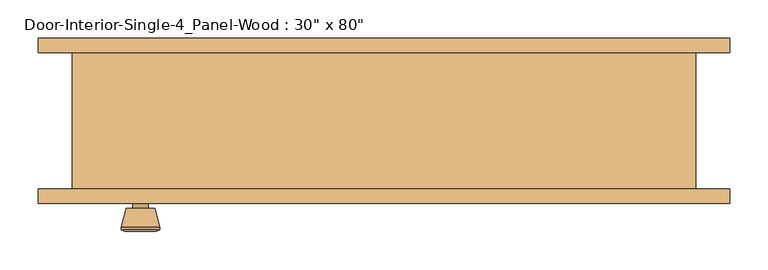
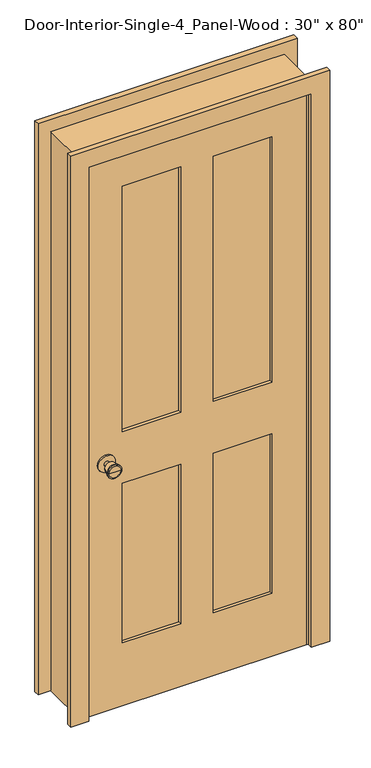
"""IFC4 building model written with IfcOpenShell, lengths in millimetres: door geometry."""

from ifc_helpers import new_model, si_unit, point, frame, frame_2d, origin, place, context, project, spatial, polyline, circle_curve, trimmed, segment, composite_curve, outline, extrude, faceted_brep, source, transform, mapped, element, save
from ifc_brep_helpers import plane_surface, cylinder_surface, revolved_surface, advanced_brep


def door_86658926(model_context):
    return source(origin(), model_context, "Body", "SolidModel", [
        advanced_brep(
        [(-317.5, -44.8, 914.4), (-327.5, -44.8, 914.4), (-307.5, -44.8, 914.4), (-297.0241324, 4.2, 914.4), (-337.9758676, 4.2, 914.4), (-317.5, 4.2, 914.4), (-292.5, 2.3721319, 914.4), (-342.5, 2.3721319, 914.4), (-292.5, -1.0915463, 914.4), (-342.5, -1.0915463, 914.4), (-298.863764, -25.8, 914.4), (-336.136236, -25.8, 914.4), (-307.5, -25.8, 914.4), (-327.5, -25.8, 914.4)],
        [
            (0, 1),
            (1, 2, circle_curve(frame((-317.5, -44.8, 914.4), z_axis=(0.0, -1.0, 0.0), x_axis=(-1.0, 0.0, 0.0)), 10.0)),
            (2, 0),
            (2, 1, circle_curve(frame((-317.5, -44.8, 914.4), z_axis=(0.0, -1.0, 0.0), x_axis=(-1.0, 0.0, 0.0)), 10.0)),
            (3, 4, circle_curve(frame((-317.5, 4.2, 914.4), z_axis=(0.0, 1.0, 0.0), x_axis=(-1.0, 0.0, 0.0)), 20.4758676)),
            (4, 5),
            (5, 3),
            (4, 3, circle_curve(frame((-317.5, 4.2, 914.4), z_axis=(0.0, 1.0, 0.0), x_axis=(-1.0, 0.0, 0.0)), 20.4758676)),
            (6, 7, circle_curve(frame((-317.5, 2.3721319, 914.4), z_axis=(0.0, 1.0, 0.0), x_axis=(-1.0, 0.0, 0.0)), 25.0)),
            (7, 4),
            (3, 6),
            (7, 6, circle_curve(frame((-317.5, 2.3721319, 914.4), z_axis=(0.0, 1.0, 0.0), x_axis=(-1.0, 0.0, 0.0)), 25.0)),
            (8, 9, circle_curve(frame((-317.5, -1.0915463, 914.4), z_axis=(0.0, 1.0, 0.0), x_axis=(-1.0, 0.0, 0.0)), 25.0)),
            (9, 7),
            (6, 8),
            (9, 8, circle_curve(frame((-317.5, -1.0915463, 914.4), z_axis=(0.0, 1.0, 0.0), x_axis=(-1.0, 0.0, 0.0)), 25.0)),
            (10, 11, circle_curve(frame((-317.5, -25.8, 914.4), z_axis=(0.0, 1.0, 0.0), x_axis=(-1.0, 0.0, 0.0)), 18.636236)),
            (11, 9),
            (8, 10),
            (11, 10, circle_curve(frame((-317.5, -25.8, 914.4), z_axis=(0.0, 1.0, 0.0), x_axis=(-1.0, 0.0, 0.0)), 18.636236)),
            (12, 13, circle_curve(frame((-317.5, -25.8, 914.4), z_axis=(0.0, 1.0, 0.0), x_axis=(-1.0, 0.0, 0.0)), 10.0)),
            (13, 11),
            (10, 12),
            (13, 12, circle_curve(frame((-317.5, -25.8, 914.4), z_axis=(0.0, 1.0, 0.0), x_axis=(-1.0, 0.0, 0.0)), 10.0)),
            (1, 13),
            (12, 2),
        ],
        [
            plane_surface(frame((-317.5, -44.8, 914.4), z_axis=(0.0, -1.0, 0.0), x_axis=(-1.0, 0.0, 0.0))),
            plane_surface(frame((-317.5, 4.2, 914.4), z_axis=(0.0, 1.0, 0.0), x_axis=(-1.0, 0.0, 0.0))),
            revolved_surface(polyline([(-337.9758676, 4.2, 914.4), (-342.5, 2.3721319, 914.4)]), (-317.5, -44.8, 914.4), (0.0, -1.0, 0.0)),
            cylinder_surface(frame((-317.5, -44.8, 914.4), z_axis=(0.0, -1.0, 0.0), x_axis=(-1.0, 0.0, 0.0)), 25.0),
            revolved_surface(polyline([(-342.5, -1.0915463, 914.4), (-336.136236, -25.8, 914.4)]), (-317.5, -44.8, 914.4), (0.0, -1.0, 0.0)),
            plane_surface(frame((-317.5, -25.8, 914.4), z_axis=(0.0, -1.0, 0.0), x_axis=(-1.0, 0.0, 0.0))),
            cylinder_surface(frame((-317.5, -44.8, 914.4), z_axis=(0.0, -1.0, 0.0), x_axis=(-1.0, 0.0, 0.0)), 10.0),
        ],
        [
            (0, [[1, 2, 3]]),
            (0, [[-3, 4, -1]]),
            (1, [[5, 6, 7]]),
            (1, [[8, -7, -6]]),
            (2, [[9, 10, -5, 11]]),
            (2, [[12, -11, -8, -10]]),
            (3, [[13, 14, -9, 15]]),
            (3, [[16, -15, -12, -14]]),
            (4, [[17, 18, -13, 19]]),
            (4, [[20, -19, -16, -18]]),
            (5, [[21, 22, -17, 23]]),
            (5, [[24, -23, -20, -22]]),
            (6, [[-2, 25, -21, 26]]),
            (6, [[-4, -26, -24, -25]]),
        ],
    ),
        extrude(outline(composite_curve([segment(trimmed(circle_curve(frame_2d((914.4, -317.5)), 30.0), [point((914.4, -347.5))], [point((914.4, -287.5))], False, "CARTESIAN"), True, "CONTINUOUS"), segment(trimmed(circle_curve(frame_2d((914.4, -317.5)), 30.0), [point((914.4, -287.5))], [point((914.4, -347.5))], False, "CARTESIAN"), True, "CONTINUOUS")], self_intersect=False)), frame((0.0, -50.8, 0.0), z_axis=(0.0, 1.0, 0.0), x_axis=(0.0, 0.0, 1.0)), (0.0, 0.0, 1.0), 6.0),
        advanced_brep(
        [(-317.5, -91.725, 914.4), (-307.5, -91.725, 914.4), (-327.5, -91.725, 914.4), (-297.0241324, -140.725, 914.4), (-317.5, -140.725, 914.4), (-337.9758676, -140.725, 914.4), (-292.5, -138.8971319, 914.4), (-342.5, -138.8971319, 914.4), (-292.5, -135.4334537, 914.4), (-342.5, -135.4334537, 914.4), (-298.863764, -110.725, 914.4), (-336.136236, -110.725, 914.4), (-307.5, -110.725, 914.4), (-327.5, -110.725, 914.4)],
        [
            (0, 1),
            (1, 2, circle_curve(frame((-317.5, -91.725, 914.4), z_axis=(0.0, 1.0, 0.0), x_axis=(-1.0, 0.0, 0.0)), 10.0)),
            (2, 0),
            (2, 1, circle_curve(frame((-317.5, -91.725, 914.4), z_axis=(0.0, 1.0, 0.0), x_axis=(-1.0, 0.0, 0.0)), 10.0)),
            (3, 4),
            (4, 5),
            (5, 3, circle_curve(frame((-317.5, -140.725, 914.4), z_axis=(0.0, -1.0, 0.0), x_axis=(-1.0, 0.0, 0.0)), 20.4758676)),
            (3, 5, circle_curve(frame((-317.5, -140.725, 914.4), z_axis=(0.0, -1.0, 0.0), x_axis=(-1.0, 0.0, 0.0)), 20.4758676)),
            (6, 3),
            (5, 7),
            (7, 6, circle_curve(frame((-317.5, -138.8971319, 914.4), z_axis=(0.0, -1.0, 0.0), x_axis=(-1.0, 0.0, 0.0)), 25.0)),
            (6, 7, circle_curve(frame((-317.5, -138.8971319, 914.4), z_axis=(0.0, -1.0, 0.0), x_axis=(-1.0, 0.0, 0.0)), 25.0)),
            (8, 6),
            (7, 9),
            (9, 8, circle_curve(frame((-317.5, -135.4334537, 914.4), z_axis=(0.0, -1.0, 0.0), x_axis=(-1.0, 0.0, 0.0)), 25.0)),
            (8, 9, circle_curve(frame((-317.5, -135.4334537, 914.4), z_axis=(0.0, -1.0, 0.0), x_axis=(-1.0, 0.0, 0.0)), 25.0)),
            (10, 8),
            (9, 11),
            (11, 10, circle_curve(frame((-317.5, -110.725, 914.4), z_axis=(0.0, -1.0, 0.0), x_axis=(-1.0, 0.0, 0.0)), 18.636236)),
            (10, 11, circle_curve(frame((-317.5, -110.725, 914.4), z_axis=(0.0, -1.0, 0.0), x_axis=(-1.0, 0.0, 0.0)), 18.636236)),
            (12, 10),
            (11, 13),
            (13, 12, circle_curve(frame((-317.5, -110.725, 914.4), z_axis=(0.0, -1.0, 0.0), x_axis=(-1.0, 0.0, 0.0)), 10.0)),
            (12, 13, circle_curve(frame((-317.5, -110.725, 914.4), z_axis=(0.0, -1.0, 0.0), x_axis=(-1.0, 0.0, 0.0)), 10.0)),
            (1, 12),
            (13, 2),
        ],
        [
            plane_surface(frame((-317.5, -91.725, 914.4), z_axis=(0.0, 1.0, 0.0), x_axis=(-1.0, 0.0, 0.0))),
            plane_surface(frame((-317.5, -140.725, 914.4), z_axis=(0.0, -1.0, 0.0), x_axis=(-1.0, 0.0, 0.0))),
            revolved_surface(polyline([(-337.9758676, -140.725, 914.4), (-342.5, -138.8971319, 914.4)]), (-317.5, -91.725, 914.4), (0.0, 1.0, 0.0)),
            cylinder_surface(frame((-317.5, -91.725, 914.4), z_axis=(0.0, 1.0, 0.0), x_axis=(-1.0, 0.0, 0.0)), 25.0),
            revolved_surface(polyline([(-342.5, -135.4334537, 914.4), (-336.136236, -110.725, 914.4)]), (-317.5, -91.725, 914.4), (0.0, 1.0, 0.0)),
            plane_surface(frame((-317.5, -110.725, 914.4), z_axis=(0.0, 1.0, 0.0), x_axis=(-1.0, 0.0, 0.0))),
            cylinder_surface(frame((-317.5, -91.725, 914.4), z_axis=(0.0, 1.0, 0.0), x_axis=(-1.0, 0.0, 0.0)), 10.0),
        ],
        [
            (0, [[1, 2, 3]]),
            (0, [[-3, 4, -1]]),
            (1, [[5, 6, 7]]),
            (1, [[-6, -5, 8]]),
            (2, [[9, -7, 10, 11]]),
            (2, [[-10, -8, -9, 12]]),
            (3, [[13, -11, 14, 15]]),
            (3, [[-14, -12, -13, 16]]),
            (4, [[17, -15, 18, 19]]),
            (4, [[-18, -16, -17, 20]]),
            (5, [[21, -19, 22, 23]]),
            (5, [[-22, -20, -21, 24]]),
            (6, [[25, -23, 26, -2]]),
            (6, [[-26, -24, -25, -4]]),
        ],
    ),
        extrude(outline(composite_curve([segment(trimmed(circle_curve(frame_2d((914.4, -317.5)), 30.0), [point((914.4, -347.5))], [point((914.4, -287.5))], False, "CARTESIAN"), True, "CONTINUOUS"), segment(trimmed(circle_curve(frame_2d((914.4, -317.5)), 30.0), [point((914.4, -287.5))], [point((914.4, -347.5))], False, "CARTESIAN"), True, "CONTINUOUS")], self_intersect=False)), frame((0.0, -91.725, 0.0), z_axis=(0.0, 1.0, 0.0), x_axis=(0.0, 0.0, 1.0)), (0.0, 0.0, 1.0), 6.0),
        extrude(outline(polyline([(260.35, -62.4416667), (260.35, -74.0833333), (57.15, -74.0833333), (57.15, -62.4416667), (260.35, -62.4416667)])), frame((0.0, 0.0, 1009.65), z_axis=(0.0, 0.0, 1.0), x_axis=(1.0, 0.0, 0.0)), (0.0, 0.0, 1.0), 903.2875),
        extrude(outline(polyline([(-57.15, -62.4416667), (-57.15, -74.0833333), (-260.35, -74.0833333), (-260.35, -62.4416667), (-57.15, -62.4416667)])), frame((0.0, 0.0, 1009.65), z_axis=(0.0, 0.0, 1.0), x_axis=(1.0, 0.0, 0.0)), (0.0, 0.0, 1.0), 903.2875),
        extrude(outline(polyline([(260.35, -62.4416667), (260.35, -74.0833333), (57.15, -74.0833333), (57.15, -62.4416667), (260.35, -62.4416667)])), frame((0.0, 0.0, 231.775), z_axis=(0.0, 0.0, 1.0), x_axis=(1.0, 0.0, 0.0)), (0.0, 0.0, 1.0), 587.375),
        extrude(outline(polyline([(-57.15, -62.4416667), (-57.15, -74.0833333), (-260.35, -74.0833333), (-260.35, -62.4416667), (-57.15, -62.4416667)])), frame((0.0, 0.0, 231.775), z_axis=(0.0, 0.0, 1.0), x_axis=(1.0, 0.0, 0.0)), (0.0, 0.0, 1.0), 587.375),
        extrude(outline(polyline([(2032.0, -381.0), (0.0, -381.0), (0.0, 381.0), (2032.0, 381.0), (2032.0, -381.0)]), holes=[polyline([(1912.9375, 57.15), (1912.9375, 260.35), (1009.65, 260.35), (1009.65, 57.15), (1912.9375, 57.15)]), polyline([(1009.65, -57.15), (1009.65, -260.35), (1912.9375, -260.35), (1912.9375, -57.15), (1009.65, -57.15)]), polyline([(819.15, 57.15), (819.15, 260.35), (231.775, 260.35), (231.775, 57.15), (819.15, 57.15)]), polyline([(231.775, -57.15), (231.775, -260.35), (819.15, -260.35), (819.15, -57.15), (231.775, -57.15)])]), frame((0.0, -85.725, 0.0), z_axis=(0.0, 1.0, 0.0), x_axis=(0.0, 0.0, 1.0)), (0.0, 0.0, 1.0), 34.925),
        faceted_brep([(406.4, -85.725, 0.0), (381.0, -85.725, 0.0), (381.0, -50.8, 0.0), (368.3, -50.8, 0.0), (368.3, -15.875, 0.0), (381.0, -15.875, 0.0), (381.0, 92.075, 0.0), (406.4, 92.075, 0.0), (406.4, 92.075, 2057.4), (406.4, -85.725, 2057.4), (381.0, 92.075, 2032.0), (-381.0, 92.075, 2032.0), (-381.0, 92.075, 0.0), (-406.4, 92.075, 0.0), (-406.4, 92.075, 2057.4), (381.0, -15.875, 2032.0), (368.3, -15.875, 2019.3), (-368.3, -15.875, 2019.3), (-368.3, -15.875, 0.0), (-381.0, -15.875, 0.0), (-381.0, -15.875, 2032.0), (368.3, -50.8, 2019.3), (381.0, -50.8, 2032.0), (-381.0, -50.8, 2032.0), (-381.0, -50.8, 0.0), (-368.3, -50.8, 0.0), (-368.3, -50.8, 2019.3), (381.0, -85.725, 2032.0), (-406.4, -85.725, 2057.4), (-406.4, -85.725, 0.0), (-381.0, -85.725, 0.0), (-381.0, -85.725, 2032.0)], [[[0, 1, 2, 3, 4, 5, 6, 7]], [[7, 8, 9, 0]], [[6, 10, 11, 12, 13, 14, 8, 7]], [[5, 15, 10, 6]], [[4, 16, 17, 18, 19, 20, 15, 5]], [[3, 21, 16, 4]], [[2, 22, 23, 24, 25, 26, 21, 3]], [[1, 27, 22, 2]], [[0, 9, 28, 29, 30, 31, 27, 1]], [[8, 14, 28, 9]], [[15, 20, 11, 10]], [[21, 26, 17, 16]], [[27, 31, 23, 22]], [[29, 13, 12, 19, 18, 25, 24, 30]], [[14, 13, 29, 28]], [[20, 19, 12, 11]], [[26, 25, 18, 17]], [[31, 30, 24, 23]]]),
        extrude(outline(polyline([(0.0, 450.85), (2101.85, 450.85), (2101.85, -450.85), (0.0, -450.85), (0.0, -387.35), (2038.35, -387.35), (2038.35, 387.35), (0.0, 387.35), (0.0, 450.85)])), frame((0.0, 92.075, 0.0), z_axis=(0.0, 1.0, 0.0), x_axis=(0.0, 0.0, 1.0)), (0.0, 0.0, 1.0), 19.05),
        extrude(outline(polyline([(0.0, 450.85), (2101.85, 450.85), (2101.85, -450.85), (0.0, -450.85), (0.0, -387.35), (2038.35, -387.35), (2038.35, 387.35), (0.0, 387.35), (0.0, 450.85)])), frame((0.0, -104.775, 0.0), z_axis=(0.0, 1.0, 0.0), x_axis=(0.0, 0.0, 1.0)), (0.0, 0.0, 1.0), 19.05),
    ])


if __name__ == "__main__":
    model = new_model("IFC4")
    model_context = context("Model", 3, world=origin())
    ifc_project = project(units=[si_unit("LENGTHUNIT", "METRE", prefix="MILLI")], contexts=[model_context])
    site = spatial("IfcSite", under=ifc_project)
    building = spatial("IfcBuilding", under=site)
    placement = place(None, origin())
    door_shape = door_86658926(model_context)
    element("IfcDoor", 1, ObjectType="Door-Interior-Single-4_Panel-Wood : 30\" x 80\"", at=placement, inside=building, context=model_context, shape_type="MappedRepresentation", body=[
        mapped(door_shape, transform((0.0, 0.0, 0.0), x_axis=(1.0, 0.0, 0.0), y_axis=(0.0, 1.0, 0.0), z_axis=(0.0, 0.0, 1.0))),
    ])
    save(model, "model.ifc")

# Revit data of these elements
# Type "Door-Interior-Single-4_Panel-Wood : 30\" x 80\""
#   Type Mark = "9"
#   Assembly Code = "C1020300"
#   Analytic Construction = "Wooden"
#   Top Rail = 0' - 4 11/16"
#   Thickness = 0' - 1 3/8"
#   Thermal Resistance (R) = 2.5876 (h·ft²·°F)/BTU
#   Swing Angle [instance default] = 90.00°
#   Stiles = 0' - 4 3/4"
#   Rough Width = 2' - 8"
#   Rough Height = 6' - 9"
#   Mullion = 0' - 4 1/2"
#   Lock Rail = 0' - 7 1/2"
#   Height = 6' - 8"
#   Width = 2' - 6"
#   Heat Transfer Coefficient (U) = 0.3865 BTU/(h·ft²·°F)
#   Bottom Rail = 0' - 9 1/8"
#   Trim Material = Cherry
#   Panel Material = Cherry
#   Frame Material = Cherry
#   Door Handle Material = Aluminum
#   Visual Light Transmittance = 0
#   Solar Heat Gain Coefficient = 0
#   Wall Closure = (empty or 0)
#   Function = (empty or 0)
# Element 1 (IfcDoor, "Door-Interior-Single-4_Panel-Wood : 30\" x 80\"")
#   Materials on its faces: "Cherry", "Aluminum"
# Materials
#   "Cherry": class "Wood", colour RGB 226 177 128, transparency 0, Description = "Prunus Serotina", Cost = 0
#   "Aluminum": class "Metal", colour RGB 247 247 247, transparency 0, Description = "Aluminum 6061", Cost = 0
